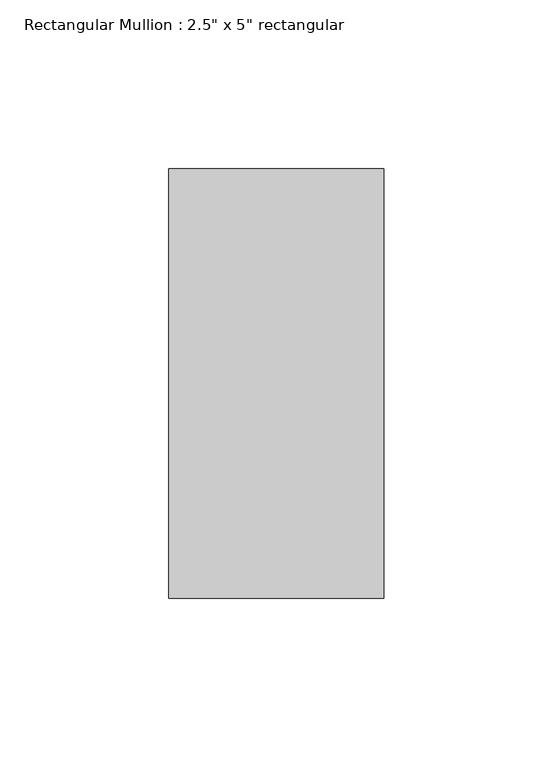
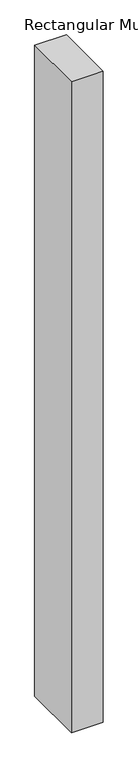
"""IFC4 building model written with IfcOpenShell, lengths in millimetres: member geometry."""

from ifc_helpers import new_model, si_unit, frame, origin, place, context, project, spatial, polyline, outline, extrude, source, transform, mapped, element, save


def member_ad4059f0(model_context):
    return source(origin(), model_context, "Body", "SweptSolid", [
        extrude(outline(polyline([(31.75, 63.5), (31.75, -63.5), (-31.75, -63.5), (-31.75, 63.5), (31.75, 63.5)])), frame((0.0, 0.0, -1375.9446538), z_axis=(0.0, 0.0, 1.0), x_axis=(1.0, 0.0, 0.0)), (0.0, 0.0, 1.0), 1375.9446538),
    ])


if __name__ == "__main__":
    model = new_model("IFC4")
    model_context = context("Model", 3, world=origin())
    ifc_project = project(units=[si_unit("LENGTHUNIT", "METRE", prefix="MILLI")], contexts=[model_context])
    site = spatial("IfcSite", under=ifc_project)
    building = spatial("IfcBuilding", under=site)
    placement = place(None, origin())
    member_shape = member_ad4059f0(model_context)
    element("IfcMember", 1, ObjectType="Rectangular Mullion : 2.5\" x 5\" rectangular", at=placement, inside=building, context=model_context, shape_type="MappedRepresentation", body=[
        mapped(member_shape, transform((0.0, 0.0, 0.0), x_axis=(1.0, 0.0, 0.0), y_axis=(0.0, 1.0, 0.0), z_axis=(0.0, 0.0, 1.0))),
    ])
    save(model, "model.ifc")

# Revit data of these elements
# Type "Rectangular Mullion : 2.5\" x 5\" rectangular"
#   built-in parameter 1007304 = 0.416667 (stored number, unit not read)
#   built-in parameter 1007301 = 0.104167 (stored number, unit not read)
#   built-in parameter 1007300 = 0.104167 (stored number, unit not read)
# Element 1 (IfcMember, "Rectangular Mullion : 2.5\" x 5\" rectangular")
#   Materials on its faces: "Aluminum"
# Materials
#   "Aluminum": class "Metal", colour RGB 247 247 247, transparency 0, Description = "Aluminum 6061", Cost = 0
